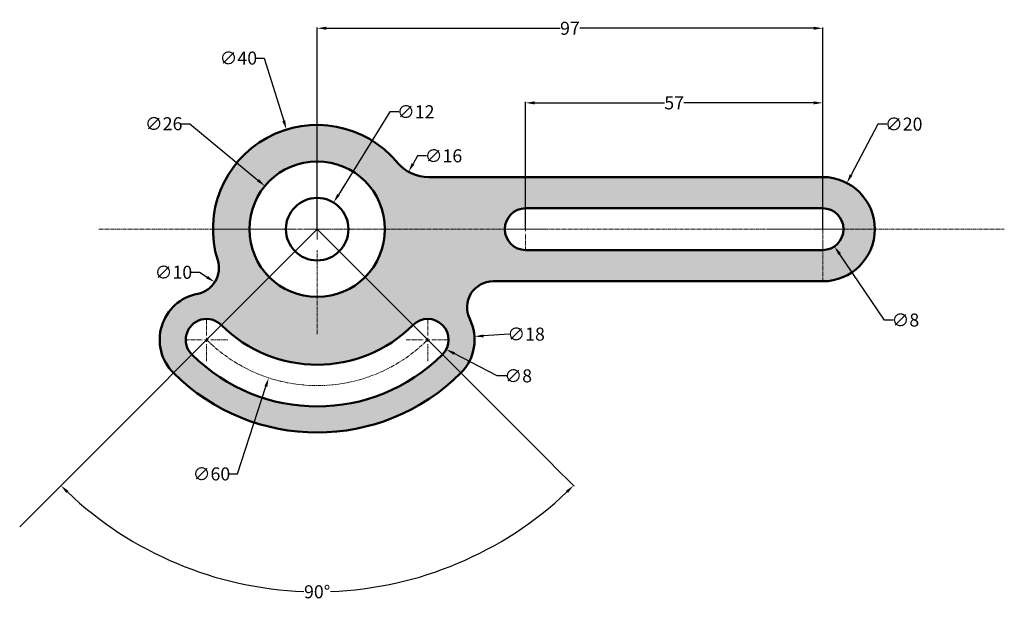
# Model space of a CAD drawing. Units: inches. Extents: x 5 to 194, y -28 to 84.
import ezdxf

# ---------------------------------------------------------------- set-up
doc = ezdxf.new("R2010")
doc.units = ezdxf.units.IN
doc.header["$MEASUREMENT"] = 0
doc.linetypes.add('CENTER2', pattern=[1.125, 0.75, -0.125, 0.125, -0.125])
for name, color, linetype, lineweight in [('M-CNTR', 4, 'CENTER2', 18), ('M-CONS', 8, 'Continuous', 13), ('M-DIMS', 2, 'Continuous', 25), ('M-OUTL', 1, 'Continuous', 50)]:
    doc.layers.add(name, color=color, linetype=linetype, lineweight=lineweight)
doc.layers.add('M-HATC', color=9, linetype='Continuous', lineweight=18, true_color=0xc7c8ca)
doc.styles.get("Standard").update_dxf_attribs({"font": 'arial.ttf'})
doc.dimstyles.get("Standard").update_dxf_attribs({"dimtxt": 2.5, "dimasz": 1.75, "dimexe": 0.18, "dimexo": 0.0625, "dimgap": 0.09, "dimtad": 0, "dimtih": 1, "dimtoh": 1, "dimdec": 0, "dimzin": 0, "dimdsep": 46, "dimtxsty": 'Standard', "dimcen": 0.09, "dimadec": 0, "dimazin": 0, "dimtfac": 1, "dimtdec": 0, "dimtofl": 0, "dimtmove": 0, "dimatfit": 3, "dimfxl": 1, "dimtolj": 1, "dimtzin": 0, "dimarcsym": 0})

# ---------------------------------------------------------------- blocks, each defined once
blk = doc.blocks.new('*D1')
at = {"layer": 'Defpoints', "color": 0, "transparency": 16777216}
for p in [(61.78, 43.34), (61.78, 43.34), (107.05, -1.93), (4.7, -13.74), (43.78, -23.85)]:
    blk.add_point(p, dxfattribs=at)
at = {"layer": 'M-DIMS', "color": 0, "lineweight": -2, "transparency": 16777216}
blk.add_line((107.09, -1.98), (111.09, -5.97), dxfattribs=at)
for start, end in [(226.4416, 267.9053), (272.0947, 313.5584)]:
    blk.add_arc((61.78, 43.34), 69.55, start, end, dxfattribs=at)
at = {"layer": 'M-DIMS', "color": 0, "transparency": 16777216}
for points in [[(13.64, -7.27), (14.05, -6.86), (12.6, -5.84)], [(109.5, -6.86), (109.91, -7.27), (110.96, -5.84)]]:
    blk.add_solid(points, dxfattribs=at)
at = {"layer": 'M-DIMS', "color": 0, "transparency": 16777216, "insert": (61.78, -26.22), "char_height": 2.5, "attachment_point": 5}
blk.add_mtext('\\A1;90°', dxfattribs=at)
blk = doc.blocks.new('*D2')
at = {"layer": 'Defpoints', "color": 0, "transparency": 16777216}
for p in [(158.78, 81.88), (61.78, 43.34), (158.78, 43.34)]:
    blk.add_point(p, dxfattribs=at)
at = {"layer": 'M-DIMS', "color": 0, "lineweight": -2, "transparency": 16777216}
for p, q in [((61.78, 43.4), (61.78, 82.06)), ((63.53, 81.88), (108.4, 81.88)), ((157.03, 81.88), (112.16, 81.88)), ((158.78, 43.4), (158.78, 82.06))]:
    blk.add_line(p, q, dxfattribs=at)
at = {"layer": 'M-DIMS', "color": 0, "transparency": 16777216}
for points in [[(63.53, 82.18), (63.53, 81.59), (61.78, 81.88)], [(157.03, 82.18), (157.03, 81.59), (158.78, 81.88)]]:
    blk.add_solid(points, dxfattribs=at)
at = {"layer": 'M-DIMS', "color": 0, "transparency": 16777216, "insert": (110.28, 81.88), "char_height": 2.5, "attachment_point": 5}
blk.add_mtext('\\A1;97', dxfattribs=at)
blk = doc.blocks.new('*D3')
at = {"layer": 'Defpoints', "color": 0, "transparency": 16777216}
for p in [(158.78, 67.57), (101.78, 43.34), (158.78, 43.34)]:
    blk.add_point(p, dxfattribs=at)
at = {"layer": 'M-DIMS', "color": 0, "lineweight": -2, "transparency": 16777216}
for p, q in [((101.78, 43.4), (101.78, 67.75)), ((103.53, 67.57), (128.4, 67.57)), ((157.03, 67.57), (132.16, 67.57)), ((158.78, 43.4), (158.78, 67.75))]:
    blk.add_line(p, q, dxfattribs=at)
at = {"layer": 'M-DIMS', "color": 0, "transparency": 16777216}
for points in [[(103.53, 67.87), (103.53, 67.28), (101.78, 67.57)], [(157.03, 67.87), (157.03, 67.28), (158.78, 67.57)]]:
    blk.add_solid(points, dxfattribs=at)
at = {"layer": 'M-DIMS', "color": 0, "transparency": 16777216, "insert": (130.28, 67.57), "char_height": 2.5, "attachment_point": 5}
blk.add_mtext('\\A1;57', dxfattribs=at)
blk = doc.blocks.new('*D4')
at = {"layer": 'Defpoints', "color": 0, "transparency": 16777216}
for p in [(55.88, 62.45), (67.68, 24.23)]:
    blk.add_point(p, dxfattribs=at)
at = {"layer": 'M-DIMS', "color": 0, "lineweight": -2, "transparency": 16777216}
for p, q in [((49.89, 76.16), (51.64, 76.16)), ((51.64, 76.16), (55.36, 64.12)), ((61.69, 43.34), (61.87, 43.34)), ((61.78, 43.25), (61.78, 43.43))]:
    blk.add_line(p, q, dxfattribs=at)
at = {"layer": 'M-DIMS', "color": 0, "transparency": 16777216}
blk.add_solid([(55.64, 64.21), (55.08, 64.03), (55.88, 62.45)], dxfattribs=at)
at = {"layer": 'M-DIMS', "color": 0, "transparency": 16777216, "insert": (46.66, 76.16), "char_height": 2.5, "attachment_point": 5}
blk.add_mtext('\\A1;∅40', dxfattribs=at)
blk = doc.blocks.new('*D5')
at = {"layer": 'Defpoints', "color": 0, "transparency": 16777216}
for p in [(51.76, 51.62), (71.8, 35.05)]:
    blk.add_point(p, dxfattribs=at)
at = {"layer": 'M-DIMS', "color": 0, "lineweight": -2, "transparency": 16777216}
for p, q in [((35.57, 63.57), (37.32, 63.57)), ((37.32, 63.57), (50.41, 52.74)), ((61.69, 43.34), (61.87, 43.34)), ((61.78, 43.25), (61.78, 43.43))]:
    blk.add_line(p, q, dxfattribs=at)
at = {"layer": 'M-DIMS', "color": 0, "transparency": 16777216}
blk.add_solid([(50.6, 52.96), (50.23, 52.51), (51.76, 51.62)], dxfattribs=at)
at = {"layer": 'M-DIMS', "color": 0, "transparency": 16777216, "insert": (32.33, 63.57), "char_height": 2.5, "attachment_point": 5}
blk.add_mtext('\\A1;∅26', dxfattribs=at)
blk = doc.blocks.new('*D6')
at = {"layer": 'Defpoints', "color": 0, "transparency": 16777216}
for p in [(64.93, 48.44), (58.62, 38.24)]:
    blk.add_point(p, dxfattribs=at)
at = {"layer": 'M-DIMS', "color": 0, "lineweight": -2, "transparency": 16777216}
for p, q in [((75.71, 65.86), (65.86, 49.93)), ((77.46, 65.86), (75.71, 65.86)), ((61.69, 43.34), (61.87, 43.34)), ((61.78, 43.25), (61.78, 43.43))]:
    blk.add_line(p, q, dxfattribs=at)
at = {"layer": 'M-DIMS', "color": 0, "transparency": 16777216}
blk.add_solid([(65.61, 50.08), (66.1, 49.77), (64.93, 48.44)], dxfattribs=at)
at = {"layer": 'M-DIMS', "color": 0, "transparency": 16777216, "insert": (80.69, 65.86), "char_height": 2.5, "attachment_point": 5}
blk.add_mtext('\\A1;∅12', dxfattribs=at)
blk = doc.blocks.new('*D7')
at = {"layer": 'Defpoints', "color": 0, "transparency": 16777216}
for p in [(79.44, 23.97), (86.54, 20.28)]:
    blk.add_point(p, dxfattribs=at)
at = {"layer": 'M-DIMS', "color": 0, "lineweight": -2, "transparency": 16777216}
for p, q in [((82.9, 22.12), (83.08, 22.12)), ((82.99, 22.03), (82.99, 22.21)), ((96.34, 15.2), (88.09, 19.48)), ((98.09, 15.2), (96.34, 15.2))]:
    blk.add_line(p, q, dxfattribs=at)
at = {"layer": 'M-DIMS', "color": 0, "transparency": 16777216}
blk.add_solid([(88.23, 19.73), (87.96, 19.22), (86.54, 20.28)], dxfattribs=at)
at = {"layer": 'M-DIMS', "color": 0, "transparency": 16777216, "insert": (100.36, 15.2), "char_height": 2.5, "attachment_point": 5}
blk.add_mtext('\\A1;∅8', dxfattribs=at)
blk = doc.blocks.new('*D8')
at = {"layer": 'Defpoints', "color": 0, "transparency": 16777216}
for p in [(91.97, 22.75), (74.01, 21.5)]:
    blk.add_point(p, dxfattribs=at)
at = {"layer": 'M-DIMS', "color": 0, "lineweight": -2, "transparency": 16777216}
for p, q in [((98.63, 23.21), (93.71, 22.87)), ((82.9, 22.12), (83.08, 22.12)), ((82.99, 22.03), (82.99, 22.21))]:
    blk.add_line(p, q, dxfattribs=at)
at = {"layer": 'M-DIMS', "color": 0, "transparency": 16777216}
blk.add_solid([(93.69, 23.16), (93.73, 22.58), (91.97, 22.75)], dxfattribs=at)
at = {"layer": 'M-DIMS', "color": 0, "transparency": 16777216, "insert": (101.87, 23.21), "char_height": 2.5, "attachment_point": 5}
blk.add_mtext('\\A1;∅18', dxfattribs=at)
blk = doc.blocks.new('*D9')
at = {"layer": 'Defpoints', "color": 0, "transparency": 16777216}
for p in [(33.7, 38.56), (42.13, 33.18)]:
    blk.add_point(p, dxfattribs=at)
at = {"layer": 'M-DIMS', "color": 0, "lineweight": -2, "transparency": 16777216}
for p, q in [((37.43, 35.07), (39.18, 35.07)), ((39.18, 35.07), (40.66, 34.12))]:
    blk.add_line(p, q, dxfattribs=at)
at = {"layer": 'M-DIMS', "color": 0, "transparency": 16777216}
blk.add_solid([(40.82, 34.37), (40.5, 33.88), (42.13, 33.18)], dxfattribs=at)
at = {"layer": 'M-DIMS', "color": 0, "transparency": 16777216, "insert": (34.2, 35.07), "char_height": 2.5, "attachment_point": 5}
blk.add_mtext('\\A1;∅10', dxfattribs=at)
blk = doc.blocks.new('*D10')
at = {"layer": 'Defpoints', "color": 0, "transparency": 16777216}
for p in [(163.42, 52.19), (154.13, 34.48)]:
    blk.add_point(p, dxfattribs=at)
at = {"layer": 'M-DIMS', "color": 0, "lineweight": -2, "transparency": 16777216}
for p, q in [((169.34, 63.49), (164.23, 53.74)), ((171.09, 63.49), (169.34, 63.49)), ((158.69, 43.34), (158.87, 43.34)), ((158.78, 43.25), (158.78, 43.43))]:
    blk.add_line(p, q, dxfattribs=at)
at = {"layer": 'M-DIMS', "color": 0, "transparency": 16777216}
blk.add_solid([(163.98, 53.88), (164.49, 53.61), (163.42, 52.19)], dxfattribs=at)
at = {"layer": 'M-DIMS', "color": 0, "transparency": 16777216, "insert": (174.33, 63.49), "char_height": 2.5, "attachment_point": 5}
blk.add_mtext('\\A1;∅20', dxfattribs=at)
blk = doc.blocks.new('*D11')
at = {"layer": 'Defpoints', "color": 0, "transparency": 16777216}
for p in [(156.53, 46.65), (161.03, 40.03)]:
    blk.add_point(p, dxfattribs=at)
at = {"layer": 'M-DIMS', "color": 0, "lineweight": -2, "transparency": 16777216}
for p, q in [((158.69, 43.34), (158.87, 43.34)), ((158.78, 43.25), (158.78, 43.43)), ((170.63, 25.91), (162.01, 38.58)), ((172.38, 25.91), (170.63, 25.91))]:
    blk.add_line(p, q, dxfattribs=at)
at = {"layer": 'M-DIMS', "color": 0, "transparency": 16777216}
blk.add_solid([(162.25, 38.75), (161.77, 38.42), (161.03, 40.03)], dxfattribs=at)
at = {"layer": 'M-DIMS', "color": 0, "transparency": 16777216, "insert": (174.65, 25.91), "char_height": 2.5, "attachment_point": 5}
blk.add_mtext('\\A1;∅8', dxfattribs=at)
blk = doc.blocks.new('*D12')
at = {"layer": 'Defpoints', "color": 0, "transparency": 16777216}
for p in [(87.13, 68.32), (79.32, 54.35)]:
    blk.add_point(p, dxfattribs=at)
at = {"layer": 'M-DIMS', "color": 0, "lineweight": -2, "transparency": 16777216}
for p, q in [((81.03, 57.41), (80.18, 55.88)), ((82.78, 57.41), (81.03, 57.41))]:
    blk.add_line(p, q, dxfattribs=at)
at = {"layer": 'M-DIMS', "color": 0, "transparency": 16777216}
blk.add_solid([(79.92, 56.02), (80.43, 55.74), (79.32, 54.35)], dxfattribs=at)
at = {"layer": 'M-DIMS', "color": 0, "transparency": 16777216, "insert": (86.02, 57.41), "char_height": 2.5, "attachment_point": 5}
blk.add_mtext('\\A1;∅16', dxfattribs=at)
blk = doc.blocks.new('*U13')
at = {"layer": 'M-CNTR', "color": 0, "transparency": 16777216}
for p, q in [((0, 0.8), (0, 4.12)), ((-4.12, 0), (-0.8, 0)), ((0.8, 0), (4.12, 0)), ((0, -4.12), (0, -0.8))]:
    blk.add_line(p, q, dxfattribs=at)
at = {"layer": 'M-CNTR', "color": 0, "linetype": 'Continuous', "transparency": 16777216}
for p, q in [((-0.4, 0), (0.4, 0)), ((0, -0.4), (0, 0.4))]:
    blk.add_line(p, q, dxfattribs=at)
blk = doc.blocks.new('*U14')
at = {"layer": 'M-CNTR', "color": 0, "transparency": 16777216}
for p, q in [((0, 0.8), (0, 4.12)), ((-4.12, 0), (-0.8, 0)), ((0.8, 0), (4.12, 0)), ((0, -4.12), (0, -0.8))]:
    blk.add_line(p, q, dxfattribs=at)
at = {"layer": 'M-CNTR', "color": 0, "linetype": 'Continuous', "transparency": 16777216}
for p, q in [((-0.4, 0), (0.4, 0)), ((0, -0.4), (0, 0.4))]:
    blk.add_line(p, q, dxfattribs=at)
blk = doc.blocks.new('*U15')
at = {"layer": 'M-CNTR', "color": 0, "transparency": 16777216}
for p, q in [((0, 4), (0, 20.12)), ((-20.12, 0), (-4, 0)), ((4, 0), (20.12, 0)), ((0, -20.12), (0, -4))]:
    blk.add_line(p, q, dxfattribs=at)
at = {"layer": 'M-CNTR', "color": 0, "linetype": 'Continuous', "transparency": 16777216}
for p, q in [((0, -2), (0, 2)), ((-2, 0), (2, 0))]:
    blk.add_line(p, q, dxfattribs=at)
blk = doc.blocks.new('*U16')
at = {"layer": 'M-CNTR', "color": 0, "transparency": 16777216}
for p, q in [((0, 0.8), (0, 4.12)), ((-4.12, 0), (-0.8, 0)), ((0.8, 0), (4.12, 0)), ((0, -4.12), (0, -0.8))]:
    blk.add_line(p, q, dxfattribs=at)
at = {"layer": 'M-CNTR', "color": 0, "linetype": 'Continuous', "transparency": 16777216}
for p, q in [((-0.4, 0), (0.4, 0)), ((0, -0.4), (0, 0.4))]:
    blk.add_line(p, q, dxfattribs=at)
blk = doc.blocks.new('*U17')
at = {"layer": 'M-CNTR', "color": 0, "transparency": 16777216}
for p, q in [((0, 0.8), (0, 4.12)), ((-4.12, 0), (-0.8, 0)), ((0.8, 0), (4.12, 0)), ((0, -4.12), (0, -0.8))]:
    blk.add_line(p, q, dxfattribs=at)
at = {"layer": 'M-CNTR', "color": 0, "linetype": 'Continuous', "transparency": 16777216}
for p, q in [((-0.4, 0), (0.4, 0)), ((0, -0.4), (0, 0.4))]:
    blk.add_line(p, q, dxfattribs=at)
blk = doc.blocks.new('*U18')
at = {"layer": 'M-CNTR', "color": 0, "transparency": 16777216}
for p, q in [((0, 2), (0, 10.12)), ((-10.12, 0), (-2, 0)), ((2, 0), (10.12, 0)), ((0, -10.12), (0, -2))]:
    blk.add_line(p, q, dxfattribs=at)
at = {"layer": 'M-CNTR', "color": 0, "linetype": 'Continuous', "transparency": 16777216}
for p, q in [((-1, 0), (1, 0)), ((0, -1), (0, 1))]:
    blk.add_line(p, q, dxfattribs=at)
blk = doc.blocks.new('*D19')
at = {"layer": 'Defpoints', "color": 0, "transparency": 16777216}
for p in [(71.07, 71.86), (52.48, 14.81)]:
    blk.add_point(p, dxfattribs=at)
at = {"layer": 'M-DIMS', "color": 0, "lineweight": -2, "transparency": 16777216}
for p, q in [((61.69, 43.34), (61.87, 43.34)), ((61.78, 43.25), (61.78, 43.43)), ((46.48, -3.61), (51.94, 13.15)), ((44.73, -3.61), (46.48, -3.61))]:
    blk.add_line(p, q, dxfattribs=at)
at = {"layer": 'M-DIMS', "color": 0, "transparency": 16777216}
blk.add_solid([(51.66, 13.24), (52.22, 13.06), (52.48, 14.81)], dxfattribs=at)
at = {"layer": 'M-DIMS', "color": 0, "transparency": 16777216, "insert": (41.5, -3.61), "char_height": 2.5, "attachment_point": 5}
blk.add_mtext('\\A1;∅60', dxfattribs=at)

msp = doc.modelspace()

# ---------------------------------------------------------------- hatches: boundary and pattern name
at = {"layer": 'M-HATC'}
h = msp.add_hatch(color=256, dxfattribs=at)
h.dxf.hatch_style = 1
h.paths.add_polyline_path([(158.78, 39.34), (101.78, 39.34, -0.414214), (97.78, 43.34), (97.66, 43.34), (74.78, 43.34, -0.198912), (70.97, 34.15), (80.16, 24.95, -1), (85.82, 19.3), (89.35, 15.76, 0.321771), (91.06, 26.12, -0.556288), (95.54, 33.34), (158.78, 33.34)])
h.paths.add_polyline_path([(158.78, 53.34), (158.78, 47.34, -0.414214), (162.78, 43.34), (168.78, 43.34, 0.414214)])
h.paths.add_polyline_path([(168.78, 43.34), (162.78, 43.34, -0.414214), (158.78, 39.34), (158.78, 33.34, 0.414214)])
h.paths.add_polyline_path([(158.78, 53.34), (83.22, 53.34, -0.221671), (77.1, 56.19, 0.221671), (61.78, 63.34), (61.78, 56.34, -0.414214), (74.78, 43.34), (81.9, 43.34), (97.78, 43.34, -0.414214), (101.78, 47.34), (158.78, 47.34)])
h.paths.add_polyline_path([(61.78, 63.34, 0.414214), (41.78, 43.34), (48.78, 43.34, -0.414214), (61.78, 56.34)])
h.paths.add_polyline_path([(48.78, 43.34), (41.78, 43.34, 0.075958), (42.69, 37.37, -0.447741), (38.86, 30.96, 0.601486), (34.2, 15.76), (37.74, 19.3, -1), (43.39, 24.95), (52.58, 34.15, -0.198912)])
h.paths.add_polyline_path([(52.58, 34.15), (43.39, 24.95, 0.414214), (80.16, 24.95), (70.97, 34.15, -0.414214)])
h.paths.add_polyline_path([(37.74, 19.3), (34.2, 15.76, 0.414214), (89.35, 15.76), (85.82, 19.3, -0.414214)])

# ---------------------------------------------------------------- linework, layer by layer
at = {"layer": 'M-CNTR'}
msp.add_line((19.9, 43.34), (193.63, 43.34), dxfattribs=at)
msp.add_arc((61.78, 43.34), 30, 225, 315, dxfattribs=at)
at = {"layer": 'M-CONS'}
for p, q in [((61.78, 43.34), (4.7, -13.74)), ((61.78, 43.34), (107.05, -1.93)), ((65.78, 39.34), (66.25, 39.34))]:
    msp.add_line(p, q, dxfattribs=at)
at = {"layer": 'M-OUTL'}
for p, q in [((83.22, 53.34), (158.78, 53.34)), ((101.78, 47.34), (158.78, 47.34)), ((101.78, 39.34), (158.78, 39.34)), ((95.54, 33.34), (158.78, 33.34))]:
    msp.add_line(p, q, dxfattribs=at)
for radius in [13, 6]:
    msp.add_circle((61.78, 43.34), radius, dxfattribs=at)
for centre, radius, start, end in [((61.78, 43.34), 20, 40.0052, 197.3748), ((83.22, 61.34), 8, 220.0052, 270), ((158.78, 43.34), 10, 270, 90), ((101.78, 43.34), 4, 90, 270), ((158.78, 43.34), 4, 270, 90), ((37.92, 35.87), 5, 280.8948, 17.3748), ((95.54, 28.34), 5, 90, 206.3466), ((40.56, 22.12), 9, 100.8948, 225), ((40.56, 22.12), 4, 44.9748, 225), ((61.78, 43.34), 26, 225.0039, 315), ((82.99, 22.12), 4, 315, 135), ((82.99, 22.12), 9, 315, 26.3466), ((61.78, 43.34), 34, 225, 315), ((61.78, 43.34), 39, 225, 315)]:
    msp.add_arc(centre, radius, start, end, dxfattribs=at)

# ---------------------------------------------------------------- block references
at = {"layer": 'M-CNTR'}
for name, p in [('*U15', (61.78, 43.34)), ('*U18', (158.78, 43.34)), ('*U16', (101.78, 43.34)), ('*U17', (158.78, 43.34)), ('*U13', (40.56, 22.12)), ('*U14', (82.99, 22.12))]:
    msp.add_blockref(name, p, dxfattribs=at)

# ---------------------------------------------------------------- dimensions: what is measured, and where the dimension line sits
at = {"layer": 'M-DIMS'}
for base, p1, picture, middle in [((158.78, 81.88), (61.78, 43.34), '*D2', (110.28, 81.88)), ((158.78, 67.57), (101.78, 43.34), '*D3', (130.28, 67.57))]:
    dim = msp.add_linear_dim(base=base, p1=p1, p2=(158.78, 43.34), dimstyle='Standard', override={"dimclrd": 0, "dimclre": 0, "dimclrt": 0}, dxfattribs=at)
    dim.commit()
    dim.dimension.update_dxf_attribs({"geometry": picture, "text_midpoint": middle})
for p1, p2, picture, middle in [((67.68, 24.23), (55.88, 62.45), '*D4', (46.66, 76.16)), ((71.07, 71.86), (52.48, 14.81), '*D19', (41.5, -3.61)), ((87.13, 68.32), (79.32, 54.35), '*D12', (86.02, 57.41)), ((58.62, 38.24), (64.93, 48.44), '*D6', (80.69, 65.86)), ((71.8, 35.05), (51.76, 51.62), '*D5', (32.33, 63.57)), ((154.13, 34.48), (163.42, 52.19), '*D10', (174.33, 63.49)), ((156.53, 46.65), (161.03, 40.03), '*D11', (174.65, 25.91)), ((33.7, 38.56), (42.13, 33.18), '*D9', (34.2, 35.07)), ((74.01, 21.5), (91.97, 22.75), '*D8', (98.63, 23.21)), ((79.44, 23.97), (86.54, 20.28), '*D7', (100.36, 15.2))]:
    dim = msp.add_diameter_dim_2p(p1=p1, p2=p2, dimstyle='Standard', override={"dimclrd": 0, "dimclre": 0, "dimclrt": 0}, dxfattribs=at)
    dim.commit()
    dim.dimension.update_dxf_attribs({"geometry": picture, "text_midpoint": middle, "dimtype": 163})
dim = msp.add_angular_dim_2l(base=(43.78, -23.85), line1=((61.78, 43.34), (107.05, -1.93)), line2=((61.78, 43.34), (4.7, -13.74)), dimstyle='Standard', override={"dimclrd": 0, "dimclre": 0, "dimclrt": 0}, dxfattribs=at)
dim.commit()
dim.dimension.update_dxf_attribs({"geometry": '*D1', "text_midpoint": (61.78, -26.22)})

doc.saveas('drawing.dxf')
